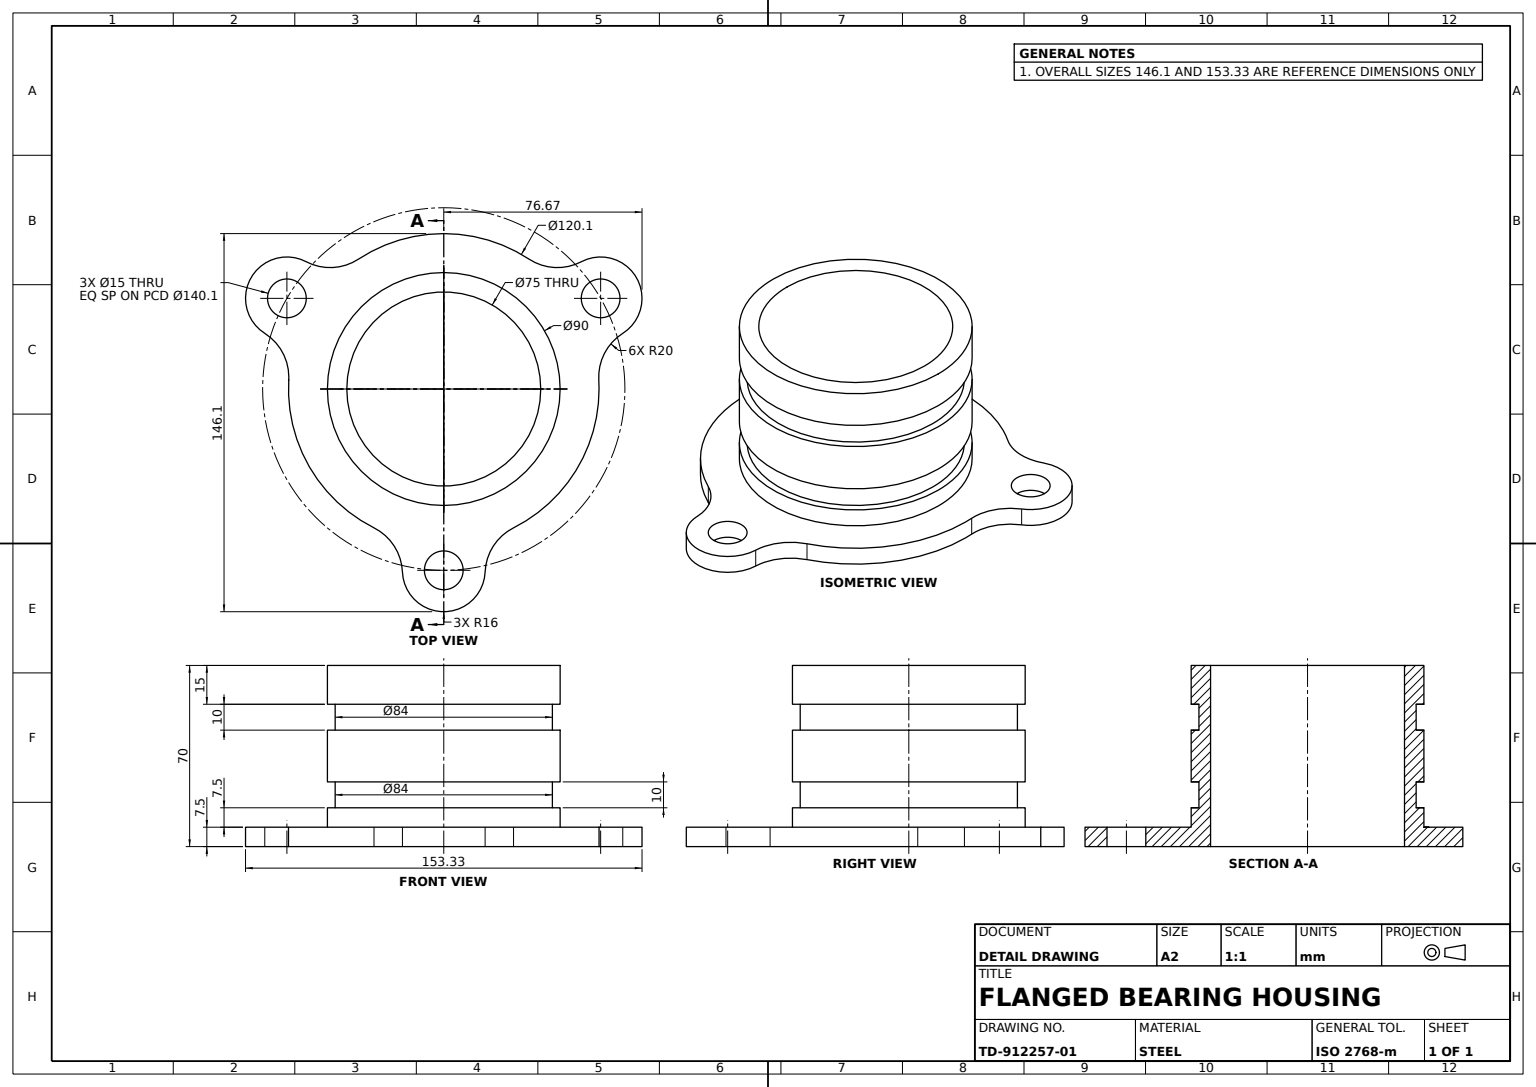
SolidWorks part; units mm, degrees
material "Plain Carbon Steel"
ref_plane "Front Plane" through (0, 0, 0) normal (0, 0, 1) x (1, 0, 0)
ref_plane "Top Plane" through (0, 0, 0) normal (0, 1, 0) x (1, 0, 0)
ref_plane "Right Plane" through (0, 0, 0) normal (1, 0, 0) x (0, 0, -1)
sketch "Housing Profile Sketch" plane through (0, 0, 0) normal (0, 0, 1) x (1, 0, 0)
  line L0 (0, -100.8944) -> (0, 100.8944) construction
  line L1 (45, 0) -> (37.5, 0)
  line L2 (37.5, 70) -> (37.5, 0)
  line L4 (45, 0) -> (45, 15)
  line L5 (45, 15) -> (42, 15)
  line L6 (42, 15) -> (42, 25)
  line L7 (42, 25) -> (45, 25)
  line L8 (45, 25) -> (45, 45)
  line L9 (45, 45) -> (42, 45)
  line L10 (42, 45) -> (42, 55)
  line L11 (42, 55) -> (45, 55)
  line L12 (45, 55) -> (45, 70)
  line L13 (45, 70) -> (37.5, 70)
  point P4 (0, 0)
  dimension "D1" = 3
  dimension "D2" = 3
  dimension "D3" = 37.5
  dimension "D4" = 45
  dimension "D5" = 45
  dimension "D6" = 70
  dimension "D7" = 15
  dimension "D8" = 15
  dimension "D9" = 10
  dimension "D10" = 20
  dimension "D11" = 7.5
revolve "Housing Sleeve Revolve" add sketch "Housing Profile Sketch" angle 360 about L0
sketch "Mounting Flange Sketch" plane through (0, 0, 0) normal (0, -1, 0) x (1, 0, 0)
  line L0 (0, -70.05) -> (0, 70.05) construction
  arc A0 (-26.9833, 53.6461) -> (-59.9505, -3.4548) centre (0, 0) ccw
  circle A1 centre (0, 0) radius 37.5 construction
  circle A2 centre (0, 0) radius 37.5
  circle A3 centre (0, 0) radius 70.05 construction
  circle A4 centre (0, 70.05) radius 7.5
  arc A6 (15.9868, 70.7003) -> (-15.9868, 70.7003) centre (0, 70.05) ccw
  arc A7 (-15.9868, 70.7003) -> (-26.9833, 53.6461) centre (-35.9703, 71.5132) cw
  arc A8 (15.9868, 70.7003) -> (26.9833, 53.6461) centre (35.9703, 71.5132) ccw
  arc A9 (53.2349, -49.1951) -> (69.2217, -21.5052) centre (60.6651, -35.025) ccw
  circle A10 centre (60.6651, -35.025) radius 7.5
  arc A11 (69.2217, -21.5052) -> (59.9505, -3.4548) centre (79.9174, -4.6055) cw
  arc A12 (53.2349, -49.1951) -> (32.9672, -50.1913) centre (43.9472, -66.9078) ccw
  arc A13 (-69.2217, -21.5052) -> (-53.2349, -49.1951) centre (-60.6651, -35.025) ccw
  circle A14 centre (-60.6651, -35.025) radius 7.5
  arc A15 (-53.2349, -49.1951) -> (-32.9672, -50.1913) centre (-43.9472, -66.9078) cw
  arc A16 (-69.2217, -21.5052) -> (-59.9505, -3.4548) centre (-79.9174, -4.6055) ccw
  arc A17 (-32.9672, -50.1913) -> (32.9672, -50.1913) centre (0, 0) ccw
  arc A18 (59.9505, -3.4548) -> (26.9833, 53.6461) centre (0, 0) ccw
  point P9 (0, 0)
  point P36 (0, 0)
  dimension "D1" = 120.1
  dimension "D2" = 140.1
  dimension "D3" = 15
  dimension "D4" = 32
  dimension "D5" = 20
  dimension "D6" = 20
  dimension "D7" = 3
extrude "Mounting Flange 3 Lugs" add sketch "Mounting Flange Sketch" against normal blind 7.5
